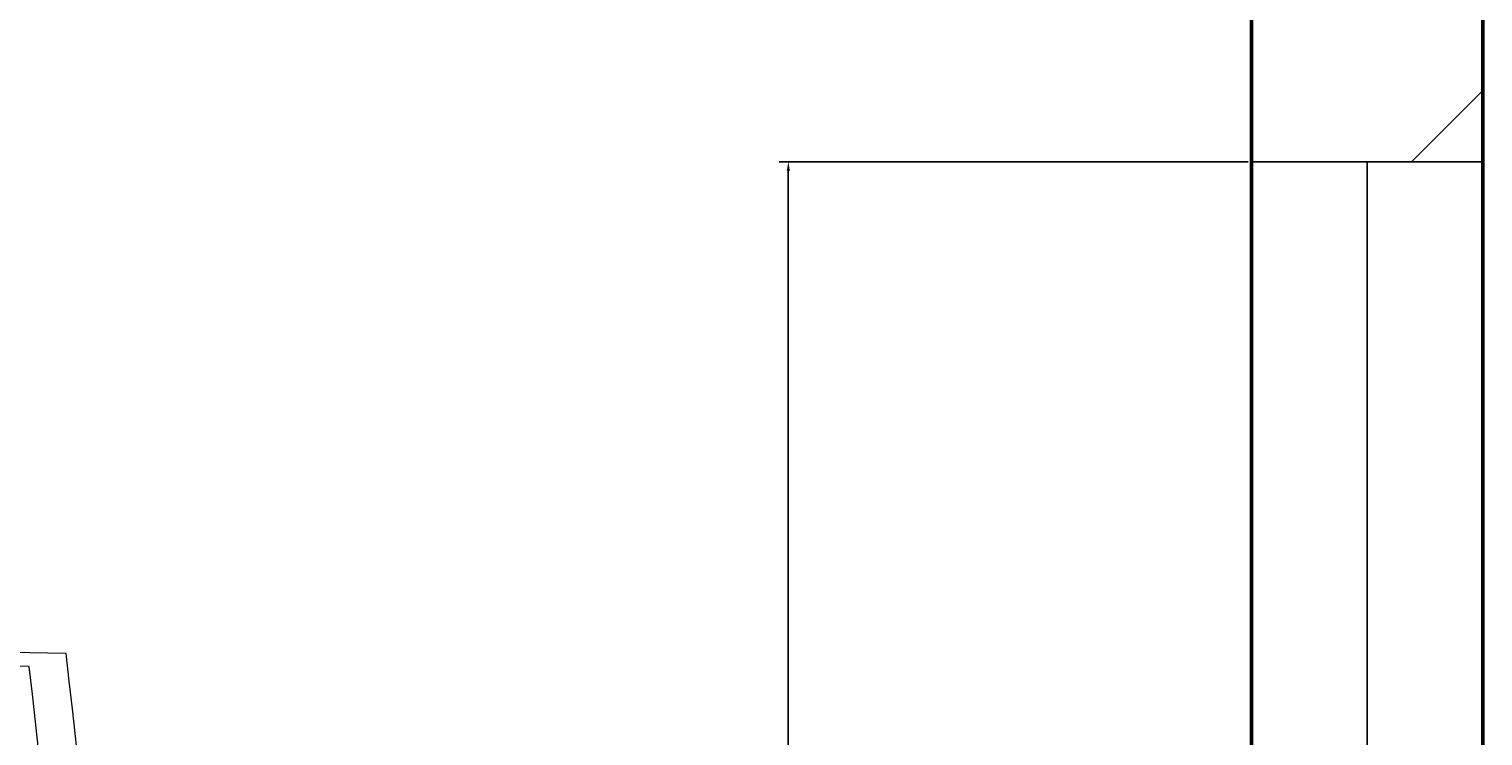
# Model space of a CAD drawing. Units: inches. Extents: x 1901 to 2863, y 888 to 2433.
# Tile 47 of 91: x 2725 to 2753, y 1622 to 1636. Entities that reach past the tile are written whole.
import ezdxf

# ---------------------------------------------------------------- set-up
doc = ezdxf.new("R2010")
doc.units = ezdxf.units.IN
for name, color, linetype, lineweight in [('A-ANNO-DIMS', 2, 'Continuous', 18), ('A-FURN', 8, 'Continuous', 18), ('A-GLAZ', 3, 'Continuous', 25), ('A-WALL', 7, 'Continuous', 50), ('A-WALL-PATT', 8, 'Continuous', 13)]:
    doc.layers.add(name, color=color, linetype=linetype, lineweight=lineweight)
doc.styles.get("Standard").update_dxf_attribs({"font": 'arial.ttf'})
doc.dimstyles.get("Standard").update_dxf_attribs({"dimtxt": 0.18, "dimasz": 0.18, "dimexe": 0.18, "dimexo": 0.0625, "dimgap": 0.09, "dimtad": 0, "dimtih": 1, "dimtoh": 1, "dimdec": 4, "dimzin": 0, "dimdsep": 46, "dimtxsty": 'Standard', "dimcen": 0.09, "dimadec": 0, "dimazin": 0, "dimtfac": 1, "dimtdec": 4, "dimtofl": 0, "dimtmove": 0, "dimatfit": 3, "dimfxl": 1, "dimtolj": 1, "dimtzin": 0, "dimarcsym": 0})

# ---------------------------------------------------------------- blocks, each defined once
blk = doc.blocks.new('BED-DOUBLE')
for centre, radius, start, end in [((205.143, 24.201), 185.219, 176.08655, 186.78213), ((205.143, 24.2), 185.219, 176.08655, 186.78213), ((204.426, 23.944), 185.219, 176.08655, 186.78213), ((204.426, 23.944), 185.219, 176.08655, 186.78213), ((23.307, 95.835), 93.531, 268.72178, 275.60397), ((22.589, 95.579), 93.531, 268.72178, 275.60397), ((22.589, 95.579), 93.531, 268.72178, 275.60397)]:
    blk.add_arc(centre, radius, start, end)
blk = doc.blocks.new('WIN-60')
for p, q in [((0, 4.5), (0, 0)), ((0, 0), (0, 2.25)), ((0, 2.25), (60, 2.25))]:
    blk.add_line(p, q)
blk = doc.blocks.new('*D19')
at = {"layer": 'A-ANNO-DIMS', "color": 0, "lineweight": -2, "transparency": 16777216}
for p, q in [((2748.364, 1633.499), (2739.246, 1633.499)), ((2739.426, 1633.319), (2739.426, 1603.682)), ((2739.426, 1573.679), (2739.426, 1603.316)), ((2748.364, 1573.499), (2739.246, 1573.499))]:
    blk.add_line(p, q, dxfattribs=at)
at = {"layer": 'A-ANNO-DIMS', "color": 0, "transparency": 16777216}
for points in [[(2739.396, 1633.319), (2739.456, 1633.319), (2739.426, 1633.499)], [(2739.396, 1573.679), (2739.456, 1573.679), (2739.426, 1573.499)]]:
    blk.add_solid(points, dxfattribs=at)
at = {"layer": 'Defpoints', "color": 0, "transparency": 16777216}
for p in [(2748.426, 1633.499), (2739.426, 1573.499), (2748.426, 1573.499)]:
    blk.add_point(p, dxfattribs=at)
at = {"layer": 'A-ANNO-DIMS', "color": 0, "transparency": 16777216, "insert": (2739.426, 1603.499), "char_height": 0.18, "attachment_point": 5}
blk.add_mtext('\\A1;WINDOW W1 60 TYP.', dxfattribs=at)

msp = doc.modelspace()

# ---------------------------------------------------------------- hatches: boundary and pattern name
at = {"layer": 'A-WALL-PATT'}
h = msp.add_hatch(dxfattribs=at)
h.set_pattern_fill('ANSI32', color=256)
h.paths.add_polyline_path([(2443.926, 2139.888), (2439.426, 2139.888), (2439.426, 2069.348), (2441.676, 2069.348), (2443.926, 2069.348), (2443.926, 2078.634), (2521.926, 2078.634), (2521.926, 2075.067), (2524.176, 2075.067), (2526.426, 2075.067), (2526.426, 2078.634), (2571.755, 2078.634), (2571.755, 2080.884), (2571.755, 2083.134), (2443.926, 2083.134)])
h.paths.add_polyline_path([(2526.426, 2054.634), (2524.176, 2054.634), (2521.926, 2054.634), (2521.926, 2030.634), (2443.926, 2030.634), (2443.926, 2045.348), (2439.426, 2045.348), (2439.426, 1983.867), (2443.926, 1983.867), (2443.926, 2026.134), (2521.926, 2026.134), (2526.426, 2026.134)])
h.paths.add_polyline_path([(2443.926, 1923.867), (2439.426, 1923.867), (2439.426, 1872.634), (2443.926, 1872.634)])
h.paths.add_polyline_path([(2636.233, 1766.134), (2609.926, 1766.134), (2609.926, 1779.785), (2605.426, 1779.785), (2605.426, 1766.134), (2486.614, 1766.134), (2486.614, 1770.671), (2482.114, 1770.671), (2482.114, 1766.134), (2482.114, 1761.634), (2636.233, 1761.634), (2636.233, 1763.884)])
h.paths.add_polyline_path([(2519.536, 1663.384), (2519.536, 1665.634), (2494.926, 1665.634), (2481.831, 1665.634), (2481.831, 1663.384), (2481.831, 1661.134), (2490.426, 1661.134), (2490.426, 1640.157), (2494.926, 1640.157), (2494.926, 1661.134), (2519.536, 1661.134)])
h.paths.add_polyline_path([(2443.926, 1712.134), (2443.926, 1716.634), (2414.464, 1716.634), (2414.464, 1712.134), (2439.426, 1712.134), (2439.426, 1545.507), (2443.926, 1545.507), (2443.926, 1661.134), (2448.475, 1661.134), (2448.475, 1665.634), (2443.926, 1665.634)])
h.paths.add_polyline_path([(2343.426, 1712.134), (2365.525, 1712.134), (2365.525, 1714.384), (2365.525, 1716.634), (2333.871, 1716.634), (2333.871, 1714.384), (2333.871, 1712.134), (2338.926, 1712.134), (2338.926, 1575.634), (2338.926, 1545.507), (2343.426, 1545.507), (2343.426, 1547.507), (2343.426, 1580.134)])
h.paths.add_polyline_path([(2752.926, 1665.634), (2579.536, 1665.634), (2579.536, 1661.134), (2615.926, 1661.134), (2615.926, 1529.134), (2598.931, 1529.134), (2598.931, 1524.634), (2623.127, 1524.634), (2623.127, 1526.884), (2623.127, 1529.134), (2620.426, 1529.134), (2620.426, 1661.134), (2748.426, 1661.134), (2748.426, 1633.499), (2752.926, 1633.499)])
h.paths.add_polyline_path([(2752.926, 1419.929), (2748.426, 1419.929), (2748.426, 1400.134), (2659.426, 1400.134), (2659.426, 1444.333), (2657.176, 1444.333), (2654.926, 1444.333), (2654.926, 1400.134), (2643.649, 1400.134), (2643.649, 1395.634), (2748.426, 1395.634), (2748.426, 1364.035), (2752.926, 1364.035)])
h.paths.add_polyline_path([(2752.926, 1492.878), (2748.426, 1492.878), (2748.426, 1476.634), (2667.426, 1476.634), (2667.426, 1479.71), (2665.176, 1479.71), (2662.926, 1479.71), (2662.926, 1476.634), (2654.926, 1476.634), (2654.926, 1469.536), (2659.426, 1469.536), (2659.426, 1472.134), (2748.426, 1472.134), (2748.426, 1455.929), (2752.926, 1455.929)])
h.paths.add_polyline_path([(2752.926, 1304.035), (2748.426, 1304.035), (2748.426, 1263.634), (2738.66, 1263.634), (2738.66, 1259.134), (2752.926, 1259.134)])
h.paths.add_polyline_path([(2685.926, 1259.134), (2695.49, 1259.134), (2695.49, 1261.384), (2695.49, 1263.634), (2677.837, 1263.634), (2677.837, 1261.384), (2677.837, 1259.134), (2681.426, 1259.134), (2681.426, 1203.634), (2653.277, 1203.634), (2653.277, 1199.134), (2685.926, 1199.134), (2685.926, 1203.634)])
h.paths.add_polyline_path([(2609.426, 1395.634), (2611.848, 1395.634), (2611.848, 1400.134), (2598.888, 1400.134), (2598.888, 1397.884), (2598.888, 1395.634), (2604.926, 1395.634), (2604.926, 1268.134), (2554.726, 1268.134), (2554.726, 1265.884), (2554.726, 1263.634), (2604.926, 1263.634), (2604.926, 1203.634), (2571.306, 1203.634), (2571.306, 1199.134), (2604.926, 1199.134), (2629.277, 1199.134), (2629.277, 1201.384), (2629.277, 1203.634), (2609.426, 1203.634), (2609.426, 1258.634), (2609.426, 1259.134), (2654.804, 1259.134), (2654.804, 1263.634), (2609.426, 1263.634)])
h.paths.add_polyline_path([(2443.926, 1304.035), (2439.426, 1304.035), (2439.426, 1259.134), (2443.926, 1259.134), (2456.16, 1259.134), (2456.16, 1261.384), (2456.16, 1263.634), (2443.926, 1263.634)])
h.paths.add_polyline_path([(2525.426, 1263.634), (2531.778, 1263.634), (2531.778, 1268.134), (2520.926, 1268.134), (2520.926, 1263.634), (2511.409, 1263.634), (2511.409, 1259.134), (2520.926, 1259.134), (2520.926, 1199.134), (2547.306, 1199.134), (2547.306, 1201.384), (2547.306, 1203.634), (2525.426, 1203.634)])
h.paths.add_polyline_path([(2443.926, 1434.842), (2439.426, 1434.842), (2439.426, 1364.035), (2441.676, 1364.035), (2443.926, 1364.035)])
h.paths.add_polyline_path([(2567.134, 1400.134), (2443.926, 1400.134), (2443.926, 1395.634), (2567.134, 1395.634)])
h.paths.add_polyline_path([(2443.926, 1545.507), (2439.426, 1545.507), (2439.426, 1494.842), (2443.926, 1494.842)])
h.paths.add_polyline_path([(2494.926, 1553.349), (2492.676, 1553.349), (2490.426, 1553.349), (2490.426, 1524.634), (2494.926, 1524.634), (2525.936, 1524.634), (2525.936, 1526.884), (2525.936, 1529.134), (2494.926, 1529.134)])
h.paths.add_polyline_path([(2752.926, 1573.499), (2748.426, 1573.499), (2748.426, 1529.134), (2657.759, 1529.134), (2657.759, 1524.634), (2662.926, 1524.634), (2662.926, 1498.631), (2667.426, 1498.631), (2667.426, 1524.634), (2748.426, 1524.634), (2748.426, 1516.878), (2752.926, 1516.878)])
h.paths.add_polyline_path([(2038.602, 2237.418), (2080.174, 2237.418), (2080.174, 2256.075), (2038.602, 2256.075)], flags=9)
h.paths.add_polyline_path([(2292.009, 1062.394), (2539.932, 1062.394), (2539.932, 1099.487), (2292.009, 1099.487)], flags=9)
h.paths.add_polyline_path([(2424.91, 1832.253), (2448.513, 1832.253), (2448.513, 1846.678), (2424.91, 1846.678)], flags=9)
h.paths.add_polyline_path([(2359.076, 1832.253), (2382.678, 1832.253), (2382.678, 1846.678), (2359.076, 1846.678)], flags=9)
h.paths.add_polyline_path([(2352.899, 1684.802), (2367.543, 1684.802), (2367.543, 1697.167), (2352.899, 1697.167)], flags=9)
h.paths.add_polyline_path([(2079.288, 1755.826), (2169.024, 1755.826), (2169.024, 1774.372), (2079.288, 1774.372)], flags=9)
h.paths.add_polyline_path([(2404.09, 1373.857), (2404.09, 1463.593), (2385.544, 1463.593), (2385.544, 1373.857)], flags=9)
h.paths.add_polyline_path([(2268.091, 2236.371), (2309.636, 2236.371), (2309.636, 2255.028), (2268.091, 2255.028)], flags=9)
h.paths.add_polyline_path([(2575.96, 1700.951), (2665.696, 1700.951), (2665.696, 1719.498), (2575.96, 1719.498)], flags=9)
h.paths.add_polyline_path([(2302.962, 1878.474), (2329.524, 1878.474), (2329.524, 1888.777), (2302.962, 1888.777)], flags=9)
h.paths.add_polyline_path([(2097.415, 2240.576), (2126.573, 2240.576), (2126.573, 2259.233), (2097.415, 2259.233)], flags=9)
h.paths.add_polyline_path([(2208.725, 2246.124), (2237.882, 2246.124), (2237.882, 2264.781), (2208.725, 2264.781)], flags=9)
h.paths.add_polyline_path([(2038.147, 1925.958), (2076.987, 1925.958), (2076.987, 1944.615), (2038.147, 1944.615)], flags=9)
h.paths.add_polyline_path([(2239.144, 1926.672), (2288.465, 1926.672), (2288.465, 1945.329), (2239.144, 1945.329)], flags=9)
h.paths.add_polyline_path([(2175.429, 2007.33), (2212.356, 2007.33), (2212.356, 2025.987), (2175.429, 2025.987)], flags=9)
h.paths.add_polyline_path([(2225.034, 2091.794), (2263.875, 2091.794), (2263.875, 2110.451), (2225.034, 2110.451)], flags=9)
h.paths.add_polyline_path([(2035.398, 2098.478), (2074.238, 2098.478), (2074.238, 2117.135), (2035.398, 2117.135)], flags=9)
h.paths.add_polyline_path([(2050.102, 2029.209), (2083.26, 2029.209), (2083.26, 2047.866), (2050.102, 2047.866)], flags=9)
h.paths.add_polyline_path([(2069.677, 1956.719), (2098.835, 1956.719), (2098.835, 1975.376), (2069.677, 1975.376)], flags=9)
h.paths.add_polyline_path([(2328.62, 1753.336), (2361.663, 1753.336), (2361.663, 1771.993), (2328.62, 1771.993)], flags=9)
h.paths.add_polyline_path([(2395.162, 2060.888), (2395.162, 2140.654), (2378.676, 2140.654), (2378.676, 2060.888)], flags=9)
h.paths.add_polyline_path([(2463.728, 2059.02), (2492.886, 2059.02), (2492.886, 2077.677), (2463.728, 2077.677)], flags=9)
h.paths.add_polyline_path([(2458.027, 2181.536), (2496.868, 2181.536), (2496.868, 2200.194), (2458.027, 2200.194)], flags=9)
h.paths.add_polyline_path([(2456.855, 2228.831), (2498.401, 2228.831), (2498.401, 2247.488), (2456.855, 2247.488)], flags=9)
h.paths.add_polyline_path([(2527.577, 2243.074), (2556.735, 2243.074), (2556.735, 2261.731), (2527.577, 2261.731)], flags=9)
h.paths.add_polyline_path([(2694.461, 2232.767), (2736.033, 2232.767), (2736.033, 2251.425), (2694.461, 2251.425)], flags=9)
h.paths.add_polyline_path([(2637.821, 2249.225), (2666.979, 2249.225), (2666.979, 2267.882), (2637.821, 2267.882)], flags=9)
h.paths.add_polyline_path([(2623.687, 2183.541), (2662.528, 2183.541), (2662.528, 2202.199), (2623.687, 2202.199)], flags=9)
h.paths.add_polyline_path([(2691.965, 2021.5), (2725.124, 2021.5), (2725.124, 2040.157), (2691.965, 2040.157)], flags=9)
h.paths.add_polyline_path([(2621.043, 1975.912), (2662.335, 1975.912), (2662.335, 1994.569), (2621.043, 1994.569)], flags=9)
h.paths.add_polyline_path([(2479.032, 1927.62), (2519.844, 1927.62), (2519.844, 1946.277), (2479.032, 1946.277)], flags=9)
h.paths.add_polyline_path([(2670.941, 1849.076), (2716.005, 1849.076), (2716.005, 1867.734), (2670.941, 1867.734)], flags=9)
h.paths.add_polyline_path([(2523.613, 1782.956), (2550.175, 1782.956), (2550.175, 1793.26), (2523.613, 1793.26)], flags=9)
h.paths.add_polyline_path([(2450.841, 1207.331), (2492.386, 1207.331), (2492.386, 1225.989), (2450.841, 1225.989)], flags=9)
h.paths.add_polyline_path([(2527.751, 1203.841), (2556.908, 1203.841), (2556.908, 1222.499), (2527.751, 1222.499)], flags=9)
h.paths.add_polyline_path([(2639.111, 1207.2), (2668.268, 1207.2), (2668.268, 1225.857), (2639.111, 1225.857)], flags=9)
h.paths.add_polyline_path([(2692.594, 1218.965), (2734.167, 1218.965), (2734.167, 1237.623), (2692.594, 1237.623)], flags=9)
h.paths.add_polyline_path([(2669.266, 1366.329), (2708.106, 1366.329), (2708.106, 1384.987), (2669.266, 1384.987)], flags=25)
h.paths.add_polyline_path([(2463.313, 1358.031), (2502.153, 1358.031), (2502.153, 1376.688), (2463.313, 1376.688)], flags=9)
h.paths.add_polyline_path([(2494.725, 1449.963), (2531.652, 1449.963), (2531.652, 1468.62), (2494.725, 1468.62)], flags=9)
h.paths.add_polyline_path([(2675.565, 1422.157), (2708.724, 1422.157), (2708.724, 1440.815), (2675.565, 1440.815)], flags=25)
h.paths.add_polyline_path([(2685.634, 1493.891), (2714.792, 1493.891), (2714.792, 1512.548), (2685.634, 1512.548)], flags=9)
h.paths.add_polyline_path([(2686.805, 1529.913), (2725.645, 1529.913), (2725.645, 1548.57), (2686.805, 1548.57)], flags=25)
h.paths.add_polyline_path([(2503.651, 1537.991), (2552.972, 1537.991), (2552.972, 1556.648), (2503.651, 1556.648)], flags=9)
h.paths.add_polyline_path([(2291.713, 1643.504), (2318.275, 1643.504), (2318.275, 1653.807), (2291.713, 1653.807)], flags=9)
h.paths.add_polyline_path([(2450.626, 1610.52), (2477.189, 1610.52), (2477.189, 1620.824), (2450.626, 1620.824)], flags=9)
h.paths.add_polyline_path([(2359.985, 1551.814), (2422.253, 1551.814), (2422.253, 1562.117), (2359.985, 1562.117)], flags=9)
h.paths.add_polyline_path([(2280.106, 1249.006), (2321.651, 1249.006), (2321.651, 1267.663), (2280.106, 1267.663)], flags=9)
h.paths.add_polyline_path([(2164.057, 1274.232), (2193.215, 1274.232), (2193.215, 1292.889), (2164.057, 1292.889)], flags=9)
h.paths.add_polyline_path([(2118.21, 1277.694), (2151.252, 1277.694), (2151.252, 1296.351), (2118.21, 1296.351)], flags=9)
h.paths.add_polyline_path([(2031.946, 1268.529), (2073.519, 1268.529), (2073.519, 1287.187), (2031.946, 1287.187)], flags=9)
h.paths.add_polyline_path([(2050.199, 1409.079), (2089.04, 1409.079), (2089.04, 1427.736), (2050.199, 1427.736)], flags=9)
h.paths.add_polyline_path([(2243.743, 1421.032), (2282.584, 1421.032), (2282.584, 1439.689), (2243.743, 1439.689)], flags=9)
h.paths.add_polyline_path([(2190.746, 1509.769), (2231.558, 1509.769), (2231.558, 1528.426), (2190.746, 1528.426)], flags=9)
h.paths.add_polyline_path([(2058.392, 1475.415), (2091.55, 1475.415), (2091.55, 1494.073), (2058.392, 1494.073)], flags=9)
h.paths.add_polyline_path([(2062.447, 1553.09), (2091.605, 1553.09), (2091.605, 1571.747), (2062.447, 1571.747)], flags=9)
h.paths.add_polyline_path([(2219.524, 1590.365), (2266.147, 1590.365), (2266.147, 1609.022), (2219.524, 1609.022)], flags=9)
h.paths.add_polyline_path([(2041.072, 1584.188), (2079.912, 1584.188), (2079.912, 1602.845), (2041.072, 1602.845)], flags=9)

# ---------------------------------------------------------------- linework, layer by layer
at = {"layer": 'A-WALL'}
for p, q in [((2752.926, 1665.634), (2752.926, 1259.134)), ((2748.426, 1661.134), (2748.426, 1529.134))]:
    msp.add_line(p, q, dxfattribs=at)

# ---------------------------------------------------------------- block references
at = {"layer": 'A-FURN', "rotation": 180}
msp.add_blockref('BED-DOUBLE', (2745.89, 1626.019), dxfattribs=at)
at = {"layer": 'A-GLAZ', "rotation": 270.0000000000013}
msp.add_blockref('WIN-60', (2748.426, 1633.5), dxfattribs=at)

# ---------------------------------------------------------------- dimensions: what is measured, and where the dimension line sits
at = {"layer": 'A-ANNO-DIMS'}
dim = msp.add_linear_dim(base=(2739.426, 1573.499), p1=(2748.426, 1633.499), p2=(2748.426, 1573.499), angle=270, text='WINDOW W1 <> TYP.', dimstyle='Standard', override={"dimdec": 0, "dimlfac": 1, "dimrnd": 0, "dimzin": 0, "dimdsep": 46, "dimlunit": 2}, dxfattribs=at)
dim.commit()
dim.dimension.update_dxf_attribs({"geometry": '*D19', "text_midpoint": (2739.426, 1603.499)})

doc.saveas('drawing.dxf')
